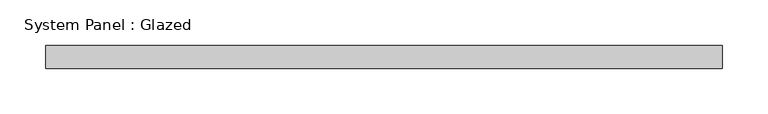
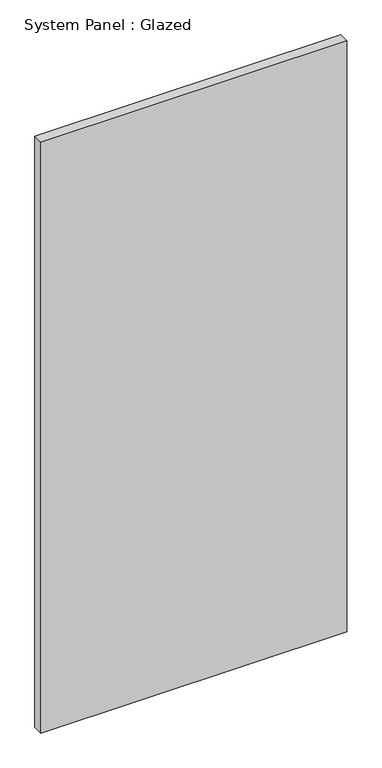
"""IFC4 building model written with IfcOpenShell, lengths in millimetres: plate geometry, System Panel : Glazed."""

from ifc_helpers import new_model, si_unit, origin, origin_with_axes, place, context, project, spatial, polyline, outline, extrude, source, transform, mapped, element, save


def system_panel_glazed_56066b17(model_context):
    return source(origin(), model_context, "Body", "SweptSolid", [
        extrude(outline(polyline([(371.475, 19.05), (-371.475, 19.05), (-371.475, 44.45), (371.475, 44.45), (371.475, 19.05)])), origin_with_axes(), (0.0, 0.0, 1.0), 1518.1858302),
    ])


if __name__ == "__main__":
    model = new_model("IFC4")
    model_context = context("Model", 3, world=origin())
    ifc_project = project(units=[si_unit("LENGTHUNIT", "METRE", prefix="MILLI")], contexts=[model_context])
    site = spatial("IfcSite", under=ifc_project)
    building = spatial("IfcBuilding", under=site)
    placement = place(None, origin())
    system_panel_glazed_shape = system_panel_glazed_56066b17(model_context)
    element("IfcPlate", 1, ObjectType="System Panel : Glazed", at=placement, inside=building, context=model_context, shape_type="MappedRepresentation", body=[
        mapped(system_panel_glazed_shape, transform((0.0, 0.0, 0.0), x_axis=(1.0, 0.0, 0.0), y_axis=(0.0, 1.0, 0.0), z_axis=(0.0, 0.0, 1.0))),
    ])
    save(model, "model.ifc")

# Revit data of these elements
# Type "System Panel : Glazed"
#   Construction Type Id = "GSP4R"
#   Analytic Construction = "1/8 in Pilkington single glazing"
#   Visual Light Transmittance = 0.9
#   Solar Heat Gain Coefficient = 0.86
#   Heat Transfer Coefficient (U) = 1.18115 BTU/(h·ft²·°F)
#   Define Thermal Properties by = 1
# Element 1 (IfcPlate, "System Panel : Glazed")
#   Materials on its faces: "Glass"
# Materials
#   "Glass": class "Glass", colour RGB 0 128 192, transparency 0.75, Description = "Soda Lime Glass", Cost = 0
